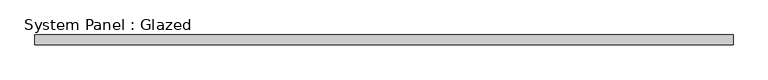
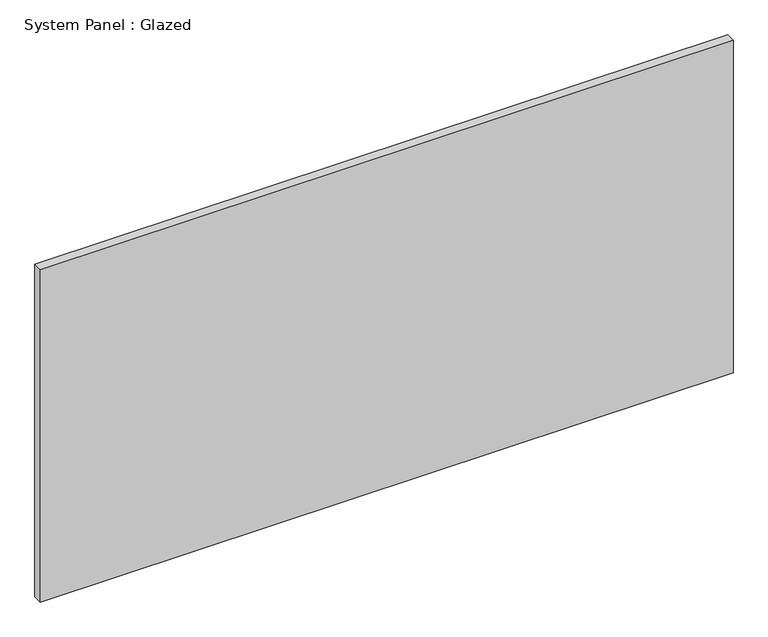
"""IFC4 building model written with IfcOpenShell, lengths in millimetres: plate geometry, System Panel : Glazed."""

from ifc_helpers import new_model, si_unit, origin, origin_with_axes, place, context, project, spatial, polyline, outline, extrude, source, transform, mapped, element, save


def system_panel_glazed_abbe3f8f(model_context):
    return source(origin(), model_context, "Body", "SweptSolid", [
        extrude(outline(polyline([(914.4, 19.05), (-914.4, 19.05), (-914.4, 44.45), (914.4, 44.45), (914.4, 19.05)])), origin_with_axes(), (0.0, 0.0, 1.0), 927.5610283),
    ])


if __name__ == "__main__":
    model = new_model("IFC4")
    model_context = context("Model", 3, world=origin())
    ifc_project = project(units=[si_unit("LENGTHUNIT", "METRE", prefix="MILLI")], contexts=[model_context])
    site = spatial("IfcSite", under=ifc_project)
    building = spatial("IfcBuilding", under=site)
    placement = place(None, origin())
    system_panel_glazed_shape = system_panel_glazed_abbe3f8f(model_context)
    element("IfcPlate", 1, ObjectType="System Panel : Glazed", at=placement, inside=building, context=model_context, shape_type="MappedRepresentation", body=[
        mapped(system_panel_glazed_shape, transform((0.0, 0.0, 0.0), x_axis=(1.0, 0.0, 0.0), y_axis=(0.0, 1.0, 0.0), z_axis=(0.0, 0.0, 1.0))),
    ])
    save(model, "model.ifc")

# Revit data of these elements
# Type "System Panel : Glazed"
#   Construction Type Id = "GSP4R"
#   Analytic Construction = "1/8 in Pilkington single glazing"
#   Visual Light Transmittance = 0.9
#   Solar Heat Gain Coefficient = 0.86
#   Heat Transfer Coefficient (U) = 1.18115 BTU/(h·ft²·°F)
# Element 1 (IfcPlate, "System Panel : Glazed")
#   Materials on its faces: "Glass"
# Materials
#   "Glass": class "Glass", colour RGB 0 128 192, transparency 0.75, Description = "Soda Lime Glass", Cost = 0
